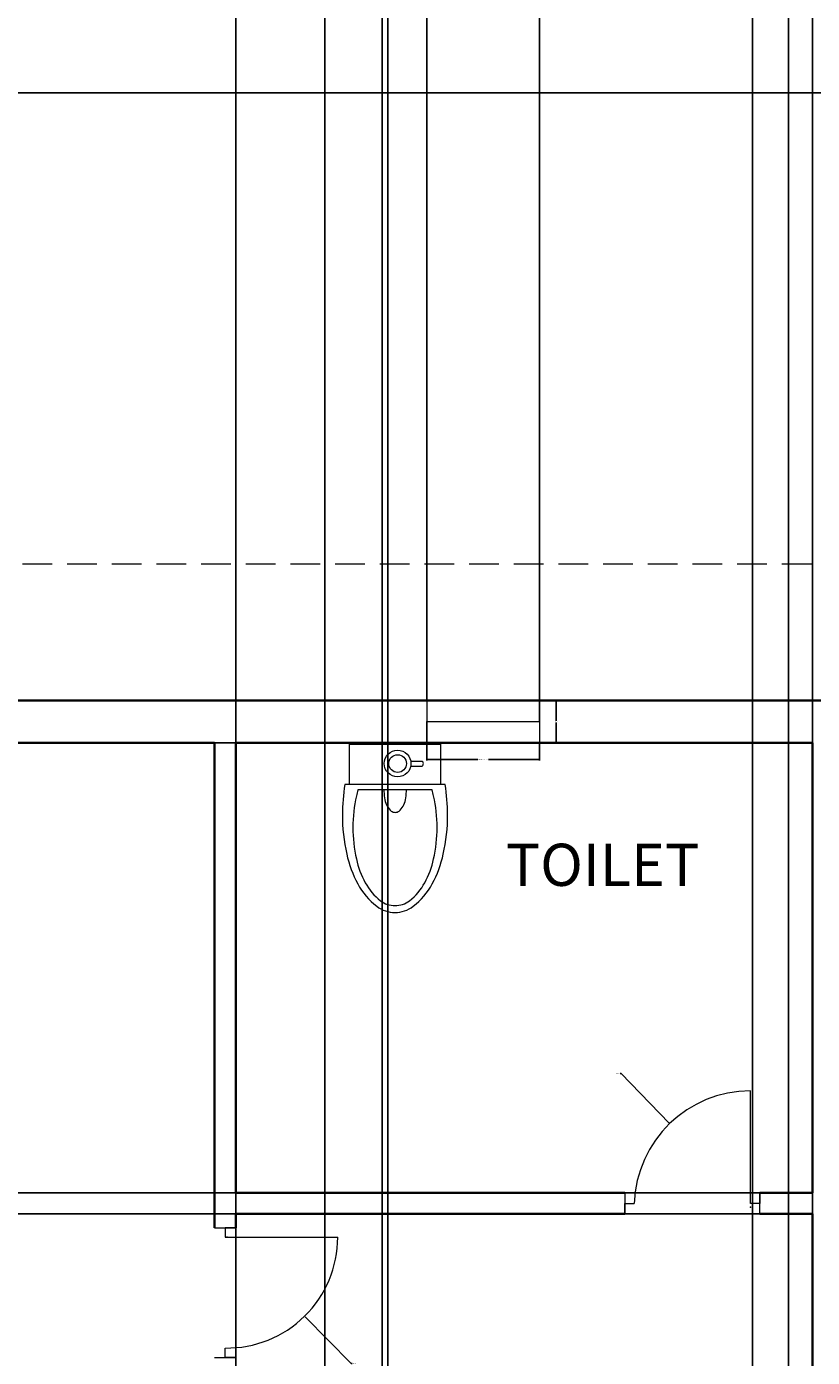
# Model space of a CAD drawing. Units: inches. Extents: x 1770 to 2988, y 1161 to 3221.
# Tile 20 of 44: x 2289 to 2456, y 2237 to 2520. Entities that reach past the tile are written whole.
import ezdxf

# ---------------------------------------------------------------- set-up
doc = ezdxf.new("R2010")
doc.units = ezdxf.units.IN
doc.linetypes.add('DASHED2', pattern=[9.525, 6.35, -3.175])
for name, color, linetype, lineweight in [('A-ANNO-DIMS', 2, 'Continuous', 18), ('A-AREA-IDEN', 7, 'Continuous', 18), ('A-DOOR', 4, 'Continuous', 18), ('A-FLOR-FIXT', 9, 'Continuous', 18), ('A-GLAZ', 4, 'Continuous', 18), ('A-ROOF-OVHD', 7, 'DASHED2', 18), ('A-WALL', 7, 'Continuous', 35), ('C-PROP', 7, 'Continuous', 25)]:
    doc.layers.add(name, color=color, linetype=linetype, lineweight=lineweight)
doc.styles.get("Standard").update_dxf_attribs({"font": 'arial.ttf'})
doc.dimstyles.get("Standard").update_dxf_attribs({"dimtxt": 0.18, "dimasz": 0.18, "dimexe": 0.18, "dimexo": 0.0625, "dimgap": 0.09, "dimtad": 0, "dimtih": 1, "dimtoh": 1, "dimdec": 4, "dimzin": 0, "dimdsep": 46, "dimtxsty": 'Standard', "dimcen": 0.09, "dimadec": 0, "dimazin": 0, "dimtfac": 1, "dimtdec": 4, "dimtofl": 0, "dimtmove": 0, "dimatfit": 3, "dimfxl": 1, "dimtolj": 1, "dimtzin": 0, "dimarcsym": 0})

# ---------------------------------------------------------------- blocks, each defined once
blk = doc.blocks.new('A$C7FD35E1A')
for p, q in [((0.0233, 0.5799), (0.0233, 0.4408)), ((0.0233, 0.5799), (0.338, 0.5799)), ((0.338, 0.5799), (0.338, 0.4408)), ((0.2357, 0.5217), (0.2745, 0.5217)), ((0.2356, 0.5044), (0.275, 0.5044)), ((0.3542, 0.4408), (0.0087, 0.4408)), ((0.3093, 0.4224), (0.0536, 0.4224))]:
    blk.add_line(p, q)
for radius in [0.046, 0.0305]:
    blk.add_circle((0.1904, 0.5132), radius)
for centre, radius, start, end in [((0.2685, 0.5129), 0.0107, 307.488, 55.394), ((0.6238, 0.337), 0.6238, 170.4184, 180), ((0.3603, 0.3321), 0.3197, 163.5954, 167.4267), ((0.277, 0.4171), 0.1337, 177.7133, 180), ((0.277, 0.4171), 0.1337, 180, 192.5399), ((0.0869, 0.4171), 0.1337, 347.4601, 0), ((0.0869, 0.4171), 0.1337, 360, 2.2867), ((0.0026, 0.3321), 0.3197, 12.5733, 16.4046), ((-0.261, 0.337), 0.6238, 0, 9.5816), ((0.5354, 0.2931), 0.4991, 167.4267, 180), ((0.23, 0.4066), 0.0855, 192.5399, 208.2349), ((0.1339, 0.4066), 0.0855, 331.7651, 347.4601), ((-0.1725, 0.2931), 0.4991, 0, 12.5733), ((0.6238, 0.337), 0.6238, 180, 192.5733), ((0.2004, 0.3907), 0.052, 208.2349, 232.3543), ((0.182, 0.3668), 0.0218, 232.3543, 270), ((0.182, 0.3668), 0.0218, 270, 307.6457), ((0.1635, 0.3907), 0.052, 307.6457, 331.7651), ((-0.261, 0.337), 0.6238, 347.4267, 0), ((0.5354, 0.2931), 0.4991, 180, 192.5733), ((-0.1725, 0.2931), 0.4991, 347.4267, 0), ((0.405, 0.2881), 0.3996, 192.5733, 208.3008), ((0.3603, 0.254), 0.3197, 192.5733, 208.3008), ((0.0026, 0.254), 0.3197, 331.6992, 347.4267), ((-0.0421, 0.2881), 0.3996, 331.6992, 347.4267), ((0.2672, 0.214), 0.2432, 208.3008, 232.4306), ((0.2501, 0.1947), 0.1945, 208.3008, 232.4306), ((0.1128, 0.1947), 0.1945, 307.5694, 331.6992), ((0.0957, 0.214), 0.2432, 307.5694, 331.6992), ((0.1814, 0.1024), 0.1024, 232.4306, 270), ((0.1814, 0.1055), 0.082, 232.4306, 270), ((0.1814, 0.1055), 0.082, 270, 307.5694), ((0.1814, 0.1024), 0.1024, 270, 307.5694)]:
    blk.add_arc(centre, radius, start, end)
blk = doc.blocks.new('WIN-24-EXT')
for p, q in [((0, 9), (0, 0)), ((24, 4.5), (24, 9)), ((24, 9), (24, 0)), ((0, 0), (0, 4.5)), ((0, 4.5), (24, 4.5))]:
    blk.add_line(p, q)
blk = doc.blocks.new('*D32')
at = {"layer": 'A-ANNO-DIMS', "color": 0, "lineweight": -2, "transparency": 16777216}
for p, q in [((2373.97, 2367.64), (2373.97, 2363.92)), ((2397.97, 2367.64), (2397.97, 2363.92)), ((2374.15, 2364.1), (2384.85, 2364.1)), ((2397.79, 2364.1), (2387.09, 2364.1))]:
    blk.add_line(p, q, dxfattribs=at)
at = {"layer": 'A-ANNO-DIMS', "color": 0, "transparency": 16777216}
for points in [[(2374.15, 2364.13), (2374.15, 2364.07), (2373.97, 2364.1)], [(2397.79, 2364.13), (2397.79, 2364.07), (2397.97, 2364.1)]]:
    blk.add_solid(points, dxfattribs=at)
at = {"layer": 'Defpoints', "color": 0, "transparency": 16777216}
for p in [(2373.97, 2367.7), (2397.97, 2367.7), (2397.97, 2364.1)]:
    blk.add_point(p, dxfattribs=at)
at = {"layer": 'A-ANNO-DIMS', "color": 0, "transparency": 16777216, "insert": (2385.97, 2364.1), "char_height": 0.18, "attachment_point": 5}
blk.add_mtext('\\A1;WINDOW 24 TYP.', dxfattribs=at)
blk = doc.blocks.new('*D33')
at = {"layer": 'A-ANNO-DIMS', "color": 0, "lineweight": -2, "transparency": 16777216}
for p, q in [((2398.03, 2376.7), (2401.75, 2376.7)), ((2401.57, 2376.52), (2401.57, 2372.38)), ((2401.57, 2367.88), (2401.57, 2372.02)), ((2398.03, 2367.7), (2401.75, 2367.7))]:
    blk.add_line(p, q, dxfattribs=at)
at = {"layer": 'A-ANNO-DIMS', "color": 0, "transparency": 16777216}
for points in [[(2401.54, 2376.52), (2401.6, 2376.52), (2401.57, 2376.7)], [(2401.54, 2367.88), (2401.6, 2367.88), (2401.57, 2367.7)]]:
    blk.add_solid(points, dxfattribs=at)
at = {"layer": 'Defpoints', "color": 0, "transparency": 16777216}
for p in [(2397.97, 2376.7), (2401.57, 2376.7), (2397.97, 2367.7)]:
    blk.add_point(p, dxfattribs=at)
at = {"layer": 'A-ANNO-DIMS', "color": 0, "transparency": 16777216, "insert": (2401.57, 2372.2), "char_height": 0.18, "attachment_point": 5}
blk.add_mtext('\\A1;9 TYP.', dxfattribs=at)
blk = doc.blocks.new('*D56')
at = {"layer": 'A-ANNO-DIMS', "color": 0, "lineweight": -2, "transparency": 16777216}
for p, q in [((1971.53, 2506.34), (1971.53, 2570.7)), ((1971.71, 2570.52), (2386.59, 2570.52)), ((2802.26, 2570.52), (2387.38, 2570.52)), ((2802.44, 2506.34), (2802.44, 2570.7))]:
    blk.add_line(p, q, dxfattribs=at)
at = {"layer": 'A-ANNO-DIMS', "color": 0, "transparency": 16777216}
for points in [[(1971.71, 2570.55), (1971.71, 2570.49), (1971.53, 2570.52)], [(2802.26, 2570.55), (2802.26, 2570.49), (2802.44, 2570.52)]]:
    blk.add_solid(points, dxfattribs=at)
at = {"layer": 'Defpoints', "color": 0, "transparency": 16777216}
for p in [(2802.44, 2570.52), (1971.53, 2506.27), (2802.44, 2506.27)]:
    blk.add_point(p, dxfattribs=at)
at = {"layer": 'A-ANNO-DIMS', "color": 0, "transparency": 16777216, "insert": (2386.99, 2570.52), "char_height": 0.18, "attachment_point": 5}
blk.add_mtext('\\A1;830.9', dxfattribs=at)
blk = doc.blocks.new('*D63')
at = {"layer": 'A-ANNO-DIMS', "color": 0, "lineweight": -2, "transparency": 16777216}
for p, q in [((2352.17, 1323.59), (2352.17, 2570.7)), ((2352.35, 2570.52), (2401.24, 2570.52)), ((2450.91, 2570.52), (2402.02, 2570.52)), ((2451.09, 1323.59), (2451.09, 2570.7))]:
    blk.add_line(p, q, dxfattribs=at)
at = {"layer": 'A-ANNO-DIMS', "color": 0, "transparency": 16777216}
for points in [[(2352.35, 2570.55), (2352.35, 2570.49), (2352.17, 2570.52)], [(2450.91, 2570.55), (2450.91, 2570.49), (2451.09, 2570.52)]]:
    blk.add_solid(points, dxfattribs=at)
at = {"layer": 'Defpoints', "color": 0, "transparency": 16777216}
for p in [(2451.09, 2570.52), (2352.17, 1323.53), (2451.09, 1323.53)]:
    blk.add_point(p, dxfattribs=at)
at = {"layer": 'A-ANNO-DIMS', "color": 0, "transparency": 16777216, "insert": (2401.63, 2570.52), "char_height": 0.18, "attachment_point": 5}
blk.add_mtext('\\A1;98.93', dxfattribs=at)
blk = doc.blocks.new('*D65')
at = {"layer": 'A-ANNO-DIMS', "color": 0, "lineweight": -2, "transparency": 16777216}
for p, q in [((2267.28, 2376.76), (2267.28, 2570.7)), ((2267.46, 2570.52), (2320.24, 2570.52)), ((2373.79, 2570.52), (2321.01, 2570.52)), ((2373.97, 2376.76), (2373.97, 2570.7))]:
    blk.add_line(p, q, dxfattribs=at)
at = {"layer": 'A-ANNO-DIMS', "color": 0, "transparency": 16777216}
for points in [[(2267.46, 2570.55), (2267.46, 2570.49), (2267.28, 2570.52)], [(2373.79, 2570.55), (2373.79, 2570.49), (2373.97, 2570.52)]]:
    blk.add_solid(points, dxfattribs=at)
at = {"layer": 'Defpoints', "color": 0, "transparency": 16777216}
for p in [(2373.97, 2570.52), (2267.28, 2376.7), (2373.97, 2376.7)]:
    blk.add_point(p, dxfattribs=at)
at = {"layer": 'A-ANNO-DIMS', "color": 0, "transparency": 16777216, "insert": (2320.62, 2570.52), "char_height": 0.18, "attachment_point": 5}
blk.add_mtext('\\A1;106.7', dxfattribs=at)
blk = doc.blocks.new('*D66')
at = {"layer": 'A-ANNO-DIMS', "color": 0, "lineweight": -2, "transparency": 16777216}
for p, q in [((2397.97, 2376.76), (2397.97, 2570.7)), ((2398.15, 2570.52), (2459.91, 2570.52)), ((2522.58, 2570.52), (2460.82, 2570.52)), ((2522.76, 2376.76), (2522.76, 2570.7))]:
    blk.add_line(p, q, dxfattribs=at)
at = {"layer": 'A-ANNO-DIMS', "color": 0, "transparency": 16777216}
for points in [[(2398.15, 2570.55), (2398.15, 2570.49), (2397.97, 2570.52)], [(2522.58, 2570.55), (2522.58, 2570.49), (2522.76, 2570.52)]]:
    blk.add_solid(points, dxfattribs=at)
at = {"layer": 'Defpoints', "color": 0, "transparency": 16777216}
for p in [(2522.76, 2570.52), (2397.97, 2376.7), (2522.76, 2376.7)]:
    blk.add_point(p, dxfattribs=at)
at = {"layer": 'A-ANNO-DIMS', "color": 0, "transparency": 16777216, "insert": (2460.36, 2570.52), "char_height": 0.18, "attachment_point": 5}
blk.add_mtext('\\A1;124.78', dxfattribs=at)
blk = doc.blocks.new('*D68')
at = {"layer": 'A-ANNO-DIMS', "color": 0, "lineweight": -2, "transparency": 16777216}
for p, q in [((2333.2, 2031.76), (2333.2, 2570.7)), ((2333.38, 2570.52), (2394.42, 2570.52)), ((2456.02, 2570.52), (2394.98, 2570.52)), ((2456.2, 2031.76), (2456.2, 2570.7))]:
    blk.add_line(p, q, dxfattribs=at)
at = {"layer": 'A-ANNO-DIMS', "color": 0, "transparency": 16777216}
for points in [[(2333.38, 2570.55), (2333.38, 2570.49), (2333.2, 2570.52)], [(2456.02, 2570.55), (2456.02, 2570.49), (2456.2, 2570.52)]]:
    blk.add_solid(points, dxfattribs=at)
at = {"layer": 'Defpoints', "color": 0, "transparency": 16777216}
for p in [(2456.2, 2570.52), (2333.2, 2031.7), (2456.2, 2031.7)]:
    blk.add_point(p, dxfattribs=at)
at = {"layer": 'A-ANNO-DIMS', "color": 0, "transparency": 16777216, "insert": (2394.7, 2570.52), "char_height": 0.18, "attachment_point": 5}
blk.add_mtext('\\A1;123', dxfattribs=at)
blk = doc.blocks.new('*D72')
at = {"layer": 'A-ANNO-DIMS', "color": 0, "lineweight": -2, "transparency": 16777216}
for p, q in [((2456.13, 2267.2), (1907.1, 2267.2)), ((1907.28, 2267.02), (1907.28, 2221.63)), ((1907.28, 2175.88), (1907.28, 2221.27)), ((2456.13, 2175.7), (1907.1, 2175.7))]:
    blk.add_line(p, q, dxfattribs=at)
at = {"layer": 'A-ANNO-DIMS', "color": 0, "transparency": 16777216}
for points in [[(1907.25, 2267.02), (1907.31, 2267.02), (1907.28, 2267.2)], [(1907.25, 2175.88), (1907.31, 2175.88), (1907.28, 2175.7)]]:
    blk.add_solid(points, dxfattribs=at)
at = {"layer": 'Defpoints', "color": 0, "transparency": 16777216}
for p in [(1907.28, 2267.2), (2456.2, 2267.2), (2456.2, 2175.7)]:
    blk.add_point(p, dxfattribs=at)
at = {"layer": 'A-ANNO-DIMS', "color": 0, "transparency": 16777216, "insert": (1907.28, 2221.45), "char_height": 0.18, "attachment_point": 5}
blk.add_mtext('\\A1;91.5', dxfattribs=at)
blk = doc.blocks.new('*D73')
at = {"layer": 'A-ANNO-DIMS', "color": 0, "lineweight": -2, "transparency": 16777216}
for p, q in [((2456.13, 2367.7), (1907.1, 2367.7)), ((1907.28, 2367.52), (1907.28, 2319.88)), ((1907.28, 2271.88), (1907.28, 2319.52)), ((2456.13, 2271.7), (1907.1, 2271.7))]:
    blk.add_line(p, q, dxfattribs=at)
at = {"layer": 'A-ANNO-DIMS', "color": 0, "transparency": 16777216}
for points in [[(1907.25, 2367.52), (1907.31, 2367.52), (1907.28, 2367.7)], [(1907.25, 2271.88), (1907.31, 2271.88), (1907.28, 2271.7)]]:
    blk.add_solid(points, dxfattribs=at)
at = {"layer": 'Defpoints', "color": 0, "transparency": 16777216}
for p in [(1907.28, 2367.7), (2456.2, 2367.7), (2456.2, 2271.7)]:
    blk.add_point(p, dxfattribs=at)
at = {"layer": 'A-ANNO-DIMS', "color": 0, "transparency": 16777216, "insert": (1907.28, 2319.7), "char_height": 0.18, "attachment_point": 5}
blk.add_mtext('\\A1;96', dxfattribs=at)
blk = doc.blocks.new('*D80')
at = {"layer": 'A-ANNO-DIMS', "color": 0, "lineweight": -2, "transparency": 16777216}
for p, q in [((2264.66, 1610.26), (2264.66, 2570.7)), ((2264.84, 2570.52), (2314.14, 2570.52)), ((2364.23, 2570.52), (2314.93, 2570.52)), ((2364.41, 1610.26), (2364.41, 2570.7))]:
    blk.add_line(p, q, dxfattribs=at)
at = {"layer": 'A-ANNO-DIMS', "color": 0, "transparency": 16777216}
for points in [[(2264.84, 2570.55), (2264.84, 2570.49), (2264.66, 2570.52)], [(2364.23, 2570.55), (2364.23, 2570.49), (2364.41, 2570.52)]]:
    blk.add_solid(points, dxfattribs=at)
at = {"layer": 'Defpoints', "color": 0, "transparency": 16777216}
for p in [(2364.41, 2570.52), (2264.66, 1610.2), (2364.41, 1610.2)]:
    blk.add_point(p, dxfattribs=at)
at = {"layer": 'A-ANNO-DIMS', "color": 0, "transparency": 16777216, "insert": (2314.53, 2570.52), "char_height": 0.18, "attachment_point": 5}
blk.add_mtext('\\A1;99.76', dxfattribs=at)
blk = doc.blocks.new('*D81')
at = {"layer": 'A-ANNO-DIMS', "color": 0, "lineweight": -2, "transparency": 16777216}
for p, q in [((2364.41, 1610.26), (2364.41, 2570.7)), ((2364.59, 2570.52), (2403.51, 2570.52)), ((2443.21, 2570.52), (2404.29, 2570.52)), ((2443.39, 1610.26), (2443.39, 2570.7))]:
    blk.add_line(p, q, dxfattribs=at)
at = {"layer": 'A-ANNO-DIMS', "color": 0, "transparency": 16777216}
for points in [[(2364.59, 2570.55), (2364.59, 2570.49), (2364.41, 2570.52)], [(2443.21, 2570.55), (2443.21, 2570.49), (2443.39, 2570.52)]]:
    blk.add_solid(points, dxfattribs=at)
at = {"layer": 'Defpoints', "color": 0, "transparency": 16777216}
for p in [(2443.39, 2570.52), (2364.41, 1610.2), (2443.39, 1610.2)]:
    blk.add_point(p, dxfattribs=at)
at = {"layer": 'A-ANNO-DIMS', "color": 0, "transparency": 16777216, "insert": (2403.9, 2570.52), "char_height": 0.18, "attachment_point": 5}
blk.add_mtext('\\A1;78.97', dxfattribs=at)
blk = doc.blocks.new('*D82')
at = {"layer": 'A-ANNO-DIMS', "color": 0, "lineweight": -2, "transparency": 16777216}
for p, q in [((2443.39, 1610.26), (2443.39, 2570.7)), ((2443.57, 2570.52), (2486.45, 2570.52)), ((2530.12, 2570.52), (2487.24, 2570.52)), ((2530.3, 1610.26), (2530.3, 2570.7))]:
    blk.add_line(p, q, dxfattribs=at)
at = {"layer": 'A-ANNO-DIMS', "color": 0, "transparency": 16777216}
for points in [[(2443.57, 2570.55), (2443.57, 2570.49), (2443.39, 2570.52)], [(2530.12, 2570.55), (2530.12, 2570.49), (2530.3, 2570.52)]]:
    blk.add_solid(points, dxfattribs=at)
at = {"layer": 'Defpoints', "color": 0, "transparency": 16777216}
for p in [(2530.3, 2570.52), (2443.39, 1610.2), (2530.3, 1610.2)]:
    blk.add_point(p, dxfattribs=at)
at = {"layer": 'A-ANNO-DIMS', "color": 0, "transparency": 16777216, "insert": (2486.85, 2570.52), "char_height": 0.18, "attachment_point": 5}
blk.add_mtext('\\A1;86.92', dxfattribs=at)
blk = doc.blocks.new('*D91')
at = {"layer": 'A-ANNO-DIMS', "color": 0, "lineweight": -2, "transparency": 16777216}
for p, q in [((2333.2, 1839.76), (2333.2, 2570.7)), ((2333.38, 2570.52), (2348.97, 2570.52)), ((2365.49, 2570.52), (2349.9, 2570.52)), ((2365.67, 1839.76), (2365.67, 2570.7))]:
    blk.add_line(p, q, dxfattribs=at)
at = {"layer": 'A-ANNO-DIMS', "color": 0, "transparency": 16777216}
for points in [[(2333.38, 2570.55), (2333.38, 2570.49), (2333.2, 2570.52)], [(2365.49, 2570.55), (2365.49, 2570.49), (2365.67, 2570.52)]]:
    blk.add_solid(points, dxfattribs=at)
at = {"layer": 'Defpoints', "color": 0, "transparency": 16777216}
for p in [(2365.67, 2570.52), (2333.2, 1839.7), (2365.67, 1839.7)]:
    blk.add_point(p, dxfattribs=at)
at = {"layer": 'A-ANNO-DIMS', "color": 0, "transparency": 16777216, "insert": (2349.43, 2570.52), "char_height": 0.18, "attachment_point": 5}
blk.add_mtext('\\A1;32.476', dxfattribs=at)
blk = doc.blocks.new('*D112')
at = {"layer": 'A-ANNO-DIMS', "color": 0, "lineweight": -2, "transparency": 16777216}
for p, q in [((2331.23, 2262.24), (2331.41, 2262.24)), ((2331.32, 2262.15), (2331.32, 2262.33)), ((2357.84, 2235.3), (2348.02, 2245.28)), ((2358.02, 2235.3), (2357.84, 2235.3))]:
    blk.add_line(p, q, dxfattribs=at)
at = {"layer": 'A-ANNO-DIMS', "color": 0, "transparency": 16777216}
blk.add_solid([(2348.04, 2245.3), (2348, 2245.26), (2347.89, 2245.41)], dxfattribs=at)
at = {"layer": 'Defpoints', "color": 0, "transparency": 16777216}
for p in [(2331.32, 2262.24), (2347.89, 2245.41)]:
    blk.add_point(p, dxfattribs=at)
at = {"layer": 'A-ANNO-DIMS', "color": 0, "transparency": 16777216, "insert": (2358.5, 2235.3), "char_height": 0.18, "attachment_point": 5}
blk.add_mtext('\\A1;R23.63', dxfattribs=at)
blk = doc.blocks.new('*D113')
at = {"layer": 'A-ANNO-DIMS', "color": 0, "lineweight": -2, "transparency": 16777216}
for p, q in [((2415.22, 2297.15), (2415.4, 2297.15)), ((2415.4, 2297.15), (2425.62, 2286.6)), ((2442.9, 2268.66), (2443.08, 2268.66)), ((2442.99, 2268.57), (2442.99, 2268.75))]:
    blk.add_line(p, q, dxfattribs=at)
at = {"layer": 'A-ANNO-DIMS', "color": 0, "transparency": 16777216}
blk.add_solid([(2425.64, 2286.62), (2425.6, 2286.58), (2425.75, 2286.47)], dxfattribs=at)
at = {"layer": 'Defpoints', "color": 0, "transparency": 16777216}
for p in [(2425.75, 2286.47), (2442.99, 2268.66)]:
    blk.add_point(p, dxfattribs=at)
at = {"layer": 'A-ANNO-DIMS', "color": 0, "transparency": 16777216, "insert": (2414.74, 2297.15), "char_height": 0.18, "attachment_point": 5}
blk.add_mtext('\\A1;R24.79', dxfattribs=at)

msp = doc.modelspace()

# ---------------------------------------------------------------- linework, layer by layer
at = {"layer": 'A-DOOR'}
for p, q in [((2442.9933, 2269.4521), (2442.9933, 2293.4521)), ((2416.2143, 2271.7021), (2416.2143, 2267.2021)), ((2444.9933, 2267.2021), (2444.9933, 2271.7021)), ((2444.9933, 2271.7021), (2444.9933, 2269.4521)), ((2416.2143, 2267.2021), (2416.2143, 2269.4521)), ((2416.2143, 2269.4521), (2418.2143, 2269.4521)), ((2444.9933, 2269.4521), (2442.9933, 2269.4521)), ((2328.696, 2264.2446), (2333.196, 2264.2446)), ((2333.196, 2264.2446), (2330.946, 2264.2446)), ((2330.946, 2264.2446), (2330.946, 2262.2446)), ((2330.946, 2262.2446), (2354.946, 2262.2446)), ((2328.696, 2236.6179), (2333.196, 2236.6179)), ((2330.946, 2236.6179), (2330.946, 2238.6179)), ((2333.196, 2236.6179), (2330.946, 2236.6179))]:
    msp.add_line(p, q, dxfattribs=at)
for centre, radius, start, end in [((2442.9933, 2268.6604), 24.7917, 90, 178.169976), ((2331.3164, 2262.2446), 23.6296, 269.101846, 0)]:
    msp.add_arc(centre, radius, start, end, dxfattribs=at)
at = {"layer": 'A-ROOF-OVHD'}
msp.add_line((2656.0216, 2405.7876), (2096.7313, 2405.7876), dxfattribs=at)
at = {"layer": 'A-WALL'}
for p, q in [((2151.696, 2376.7021), (2625.696, 2376.7021)), ((2160.696, 2367.7021), (2328.696, 2367.7021)), ((2328.696, 2367.7021), (2328.696, 2264.2446)), ((2333.196, 2367.7021), (2333.196, 2271.7021)), ((2333.196, 2367.7021), (2333.196, 2271.7021)), ((2333.196, 2367.7021), (2456.196, 2367.7021)), ((2456.196, 2367.7021), (2456.196, 2271.7021)), ((2333.196, 2271.7021), (2416.2143, 2271.7021)), ((2444.9933, 2271.7021), (2456.196, 2271.7021)), ((2333.196, 2267.2021), (2333.196, 2264.2446)), ((2416.2143, 2267.2021), (2333.196, 2267.2021)), ((2456.196, 2267.2021), (2444.9933, 2267.2021)), ((2456.196, 2267.2021), (2456.196, 2175.7021))]:
    msp.add_line(p, q, dxfattribs=at)
at = {"layer": 'C-PROP'}
msp.add_lwpolyline([(1971.5344, 2506.2747), (2802.4374, 2506.2747), (2802.4374, 1323.5288), (1971.5344, 1323.5288)], close=True, dxfattribs=at)

# ---------------------------------------------------------------- block references
at = {"layer": 'A-FLOR-FIXT', "xscale": 61.88350044382122, "yscale": 61.88350044382122, "zscale": 61.88350044382122}
msp.add_blockref('A$C7FD35E1A', (2355.9409, 2331.5017), dxfattribs=at)
at = {"layer": 'A-GLAZ'}
msp.add_blockref('WIN-24-EXT', (2373.971, 2367.702), dxfattribs=at)

# ---------------------------------------------------------------- texts
at = {"layer": 'A-AREA-IDEN', "insert": (2390.7826, 2346.1664), "char_height": 9, "attachment_point": 1}
msp.add_mtext_dynamic_manual_height_columns('TOILET', width=83.344593, gutter_width=12.5, heights=[0], dxfattribs=at)

# ---------------------------------------------------------------- dimensions: what is measured, and where the dimension line sits
at = {"layer": 'A-ANNO-DIMS'}
for base, p1, p2, override, picture, middle in [((2802.4374, 2570.5247), (1971.5344, 2506.2747), (2802.4374, 2506.2747), {"dimdec": 1, "dimlfac": 1, "dimrnd": 0, "dimzin": 0, "dimdsep": 46, "dimlunit": 2}, '*D56', (2386.9859, 2570.5247)), ((2364.4122, 2570.5247), (2264.6568, 1610.2021), (2364.4122, 1610.2021), {"dimdec": 2, "dimlfac": 1, "dimrnd": 0, "dimzin": 0, "dimdsep": 46, "dimlunit": 2}, '*D80', (2314.5345, 2570.5247)), ((2373.9714, 2570.5247), (2267.2776, 2376.7021), (2373.9714, 2376.7021), {"dimdec": 1, "dimlfac": 1, "dimrnd": 0, "dimzin": 0, "dimdsep": 46, "dimlunit": 2}, '*D65', (2320.6245, 2570.5247)), ((2456.196, 2570.5247), (2333.196, 2031.7021), (2456.196, 2031.7021), {"dimdec": 0, "dimlfac": 1, "dimrnd": 0, "dimzin": 0, "dimdsep": 46, "dimlunit": 2}, '*D68', (2394.696, 2570.5247)), ((2365.672, 2570.5247), (2333.196, 1839.7021), (2365.672, 1839.7021), {"dimdec": 3, "dimlfac": 1, "dimrnd": 0, "dimzin": 0, "dimdsep": 46, "dimlunit": 2}, '*D91', (2349.434, 2570.5247)), ((2451.0947, 2570.5247), (2352.1672, 1323.5288), (2451.0947, 1323.5288), {"dimdec": 2, "dimlfac": 1, "dimrnd": 0, "dimzin": 0, "dimdsep": 46, "dimlunit": 2}, '*D63', (2401.631, 2570.5247)), ((2443.3863, 2570.5247), (2364.4122, 1610.2021), (2443.3863, 1610.2021), {"dimdec": 2, "dimlfac": 1, "dimrnd": 0, "dimzin": 0, "dimdsep": 46, "dimlunit": 2}, '*D81', (2403.8993, 2570.5247)), ((2522.7552, 2570.5247), (2397.9714, 2376.7021), (2522.7552, 2376.7021), {"dimdec": 2, "dimlfac": 1, "dimrnd": 0, "dimzin": 0, "dimdsep": 46, "dimlunit": 2}, '*D66', (2460.3633, 2570.5247)), ((2530.3038, 2570.5247), (2443.3863, 1610.2021), (2530.3038, 1610.2021), {"dimdec": 2, "dimlfac": 1, "dimrnd": 0, "dimzin": 0, "dimdsep": 46, "dimlunit": 2}, '*D82', (2486.8451, 2570.5247))]:
    dim = msp.add_linear_dim(base=base, p1=p1, p2=p2, dimstyle='Standard', override=override, dxfattribs=at)
    dim.commit()
    dim.dimension.update_dxf_attribs({"geometry": picture, "text_midpoint": middle})
dim = msp.add_linear_dim(base=(2401.5714, 2376.7021), p1=(2397.9714, 2367.7021), p2=(2397.9714, 2376.7021), angle=90, text='<> TYP.', dimstyle='Standard', override={"dimdec": 0, "dimlfac": 1, "dimrnd": 0, "dimzin": 0, "dimdsep": 46, "dimlunit": 2}, dxfattribs=at)
dim.commit()
dim.dimension.update_dxf_attribs({"geometry": '*D33', "text_midpoint": (2401.5714, 2372.2021)})
for base, p1, p2, override, picture, middle in [((1907.2844, 2367.7021), (2456.196, 2271.7021), (2456.196, 2367.7021), {"dimdec": 0, "dimlfac": 1, "dimrnd": 0, "dimzin": 0, "dimdsep": 46, "dimlunit": 2}, '*D73', (1907.2844, 2319.7021)), ((1907.2844, 2267.2021), (2456.196, 2175.7021), (2456.196, 2267.2021), {"dimdec": 1, "dimlfac": 1, "dimrnd": 0, "dimzin": 0, "dimdsep": 46, "dimlunit": 2}, '*D72', (1907.2844, 2221.4521))]:
    dim = msp.add_linear_dim(base=base, p1=p1, p2=p2, angle=90, dimstyle='Standard', override=override, dxfattribs=at)
    dim.commit()
    dim.dimension.update_dxf_attribs({"geometry": picture, "text_midpoint": middle})
dim = msp.add_linear_dim(base=(2397.9714, 2364.1021), p1=(2373.9714, 2367.7021), p2=(2397.9714, 2367.7021), text='WINDOW <> TYP.', dimstyle='Standard', override={"dimdec": 0, "dimlfac": 1, "dimrnd": 0, "dimzin": 0, "dimdsep": 46, "dimlunit": 2}, dxfattribs=at)
dim.commit()
dim.dimension.update_dxf_attribs({"geometry": '*D32', "text_midpoint": (2385.9714, 2364.1021)})
for center, mpoint, picture, middle in [((2442.9933, 2268.6604), (2425.7453, 2286.4687), '*D113', (2414.7365, 2297.1537)), ((2331.3164, 2262.2446), (2347.894, 2245.406), '*D112', (2358.5004, 2235.3028))]:
    dim = msp.add_radius_dim(center=center, mpoint=mpoint, dimstyle='Standard', override={"dimdec": 2, "dimlfac": 1, "dimrnd": 0, "dimzin": 0, "dimdsep": 46, "dimlunit": 2}, dxfattribs=at)
    dim.commit()
    dim.dimension.update_dxf_attribs({"geometry": picture, "text_midpoint": middle, "dimtype": 164})

doc.saveas('drawing.dxf')
